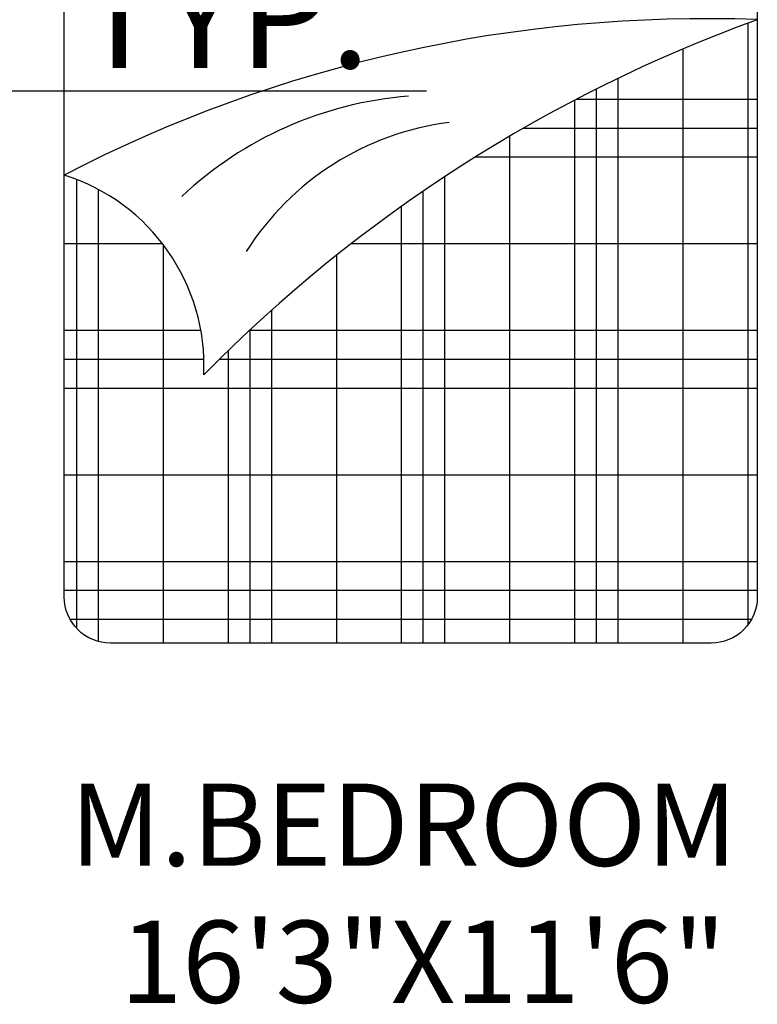
# Model space of a CAD drawing. Units: inches. Extents: x 3064 to 19385, y 846 to 15425.
# Tile 6 of 108: x 3426 to 3489, y 1289 to 1373. Entities that reach past the tile are written whole.
import ezdxf

# ---------------------------------------------------------------- set-up
doc = ezdxf.new("R2010")
doc.units = ezdxf.units.IN
for name, color, linetype, lineweight in [('A-ANNO-DIMS', 2, 'Continuous', 18), ('A-AREA-IDEN', 3, 'Continuous', 18), ('A-FLOR-FIXT', 9, 'Continuous', 18)]:
    doc.layers.add(name, color=color, linetype=linetype, lineweight=lineweight)
doc.layers.add('BLOCK', color=6, linetype='Continuous')
doc.styles.get("Standard").update_dxf_attribs({"font": 'arial.ttf'})
doc.dimstyles.new('ISO-25', dxfattribs={"dimtxt": 9, "dimasz": 2.5, "dimexe": 1.25, "dimexo": 0.625, "dimtad": 1, "dimdec": 1, "dimlunit": 3, "dimtxsty": 'Standard', "dimcen": 2.5, "dimadec": 0, "dimazin": 0, "dimtfac": 1, "dimtdec": 1, "dimtmove": 0, "dimatfit": 3, "dimfxl": 1, "dimarcsym": 0})

# ---------------------------------------------------------------- blocks, each defined once
blk = doc.blocks.new('*X5')
at = {"color": 0}
for p, q in [((276.598, 451.25), (280.51, 451.25)), ((275.455, 450.625), (280.51, 450.625)), ((274.411, 450), (280.51, 450)), ((265.51, 448.125), (267.634, 448.125)), ((271.723, 448.125), (280.51, 448.125)), ((265.51, 446.25), (268.465, 446.25)), ((269.519, 446.25), (280.51, 446.25)), ((265.51, 445.625), (268.531, 445.625)), ((268.866, 445.625), (280.51, 445.625)), ((265.51, 445), (280.51, 445)), ((265.51, 443.125), (280.51, 443.125)), ((265.51, 441.25), (280.51, 441.25)), ((265.51, 440.625), (280.51, 440.625)), ((265.634, 440), (280.386, 440))]:
    blk.add_line(p, q, dxfattribs=at)
blk = doc.blocks.new('*X6')
at = {"color": 0}
for p, q in [((280.312, 439.886), (280.312, 452.896)), ((278.906, 439.482), (278.906, 452.338)), ((277.5, 439.482), (277.5, 451.702)), ((277.031, 439.482), (277.031, 451.471)), ((276.562, 439.482), (276.562, 451.231)), ((275.156, 439.482), (275.156, 450.451)), ((265.781, 439.797), (265.781, 449.511)), ((273.75, 439.482), (273.75, 449.576)), ((266.25, 439.517), (266.25, 449.296)), ((273.281, 439.482), (273.281, 449.261)), ((272.812, 439.482), (272.812, 448.934)), ((267.656, 439.482), (267.656, 448.095)), ((271.406, 439.482), (271.406, 447.876)), ((270, 439.482), (270, 446.689)), ((269.531, 439.482), (269.531, 446.262)), ((269.062, 439.482), (269.062, 445.817))]:
    blk.add_line(p, q, dxfattribs=at)
blk = doc.blocks.new('A$C52E67D0D')
at = {"layer": 'BLOCK'}
blk.add_lwpolyline([(1901, 0), (601, 0, -0.414214), (501, 100), (501, 1700, -0.414214), (601, 1800), (1901, 1800, -0.414214), (2001, 1700), (2001, 100, -0.414214)], format="xyb", close=True, dxfattribs=at)
for centre, radius, start, end in [((1888.6, -1664.5), 3015.3, 87.8642, 117.4001), ((3101, -1685.8), 3227.7, 109.926, 135.3977), ((1308.8, 377.9), 807.6, 94.4436, 133.2788), ((1410.8, 520.2), 610.8, 97.2157, 147.6656), ((371.4, 600.4), 432, 357.3792, 72.5379)]:
    blk.add_arc(centre, radius, start, end, dxfattribs=at)
at = {"layer": 'BLOCK', "xscale": 100, "yscale": 100, "zscale": 100}
for name in ['*X6', '*X5']:
    blk.add_blockref(name, (-26050, -43948.2), dxfattribs=at)
blk = doc.blocks.new('*D427')
at = {"layer": 'A-ANNO-DIMS', "color": 0, "lineweight": -2, "transparency": 16777216}
for p, q in [((3296.059, 1369.474), (3296.059, 1365.249)), ((3320.059, 1369.474), (3320.059, 1365.249)), ((3298.559, 1366.499), (3317.559, 1366.499)), ((3320.059, 1366.499), (3460.682, 1366.499))]:
    blk.add_line(p, q, dxfattribs=at)
at = {"layer": 'A-ANNO-DIMS', "color": 0, "transparency": 16777216}
for points in [[(3298.559, 1366.915), (3298.559, 1366.082), (3296.059, 1366.499)], [(3317.559, 1366.915), (3317.559, 1366.082), (3320.059, 1366.499)]]:
    blk.add_solid(points, dxfattribs=at)
at = {"layer": 'Defpoints', "color": 0, "transparency": 16777216}
for p in [(3296.059, 1370.099), (3320.059, 1370.099), (3320.059, 1366.499)]:
    blk.add_point(p, dxfattribs=at)
at = {"layer": 'A-ANNO-DIMS', "color": 0, "transparency": 16777216, "insert": (3391.621, 1371.78), "char_height": 9, "attachment_point": 5}
blk.add_mtext('MICROWAVE 2\'-0" TYP.', dxfattribs=at)

msp = doc.modelspace()

# ---------------------------------------------------------------- block references
at = {"layer": 'A-FLOR-FIXT', "xscale": 0.039370099999992, "yscale": 0.039370099999992, "zscale": 0.039370099999992}
msp.add_blockref('A$C52E67D0D', (3410.096, 1319.474), dxfattribs=at)

# ---------------------------------------------------------------- texts
at = {"layer": 'A-AREA-IDEN', "insert": (3430.297, 1307.513), "char_height": 7, "attachment_point": 1}
msp.add_mtext_dynamic_manual_height_columns('M.BEDROOM\\P  16\'3"X11\'6"', width=67.59241, gutter_width=12.5, heights=[0], dxfattribs=at)

# ---------------------------------------------------------------- dimensions: what is measured, and where the dimension line sits
at = {"layer": 'A-ANNO-DIMS'}
dim = msp.add_linear_dim(base=(3320.059, 1366.499), p1=(3296.059, 1370.099), p2=(3320.059, 1370.099), text='MICROWAVE <> TYP.', dimstyle='ISO-25', override={"dimdec": 1, "dimrnd": 0, "dimzin": 1, "dimlunit": 4, "dimfrac": 2}, dxfattribs=at)
dim.commit()
dim.dimension.update_dxf_attribs({"geometry": '*D427', "text_midpoint": (3391.621, 1371.78)})

doc.saveas('drawing.dxf')
